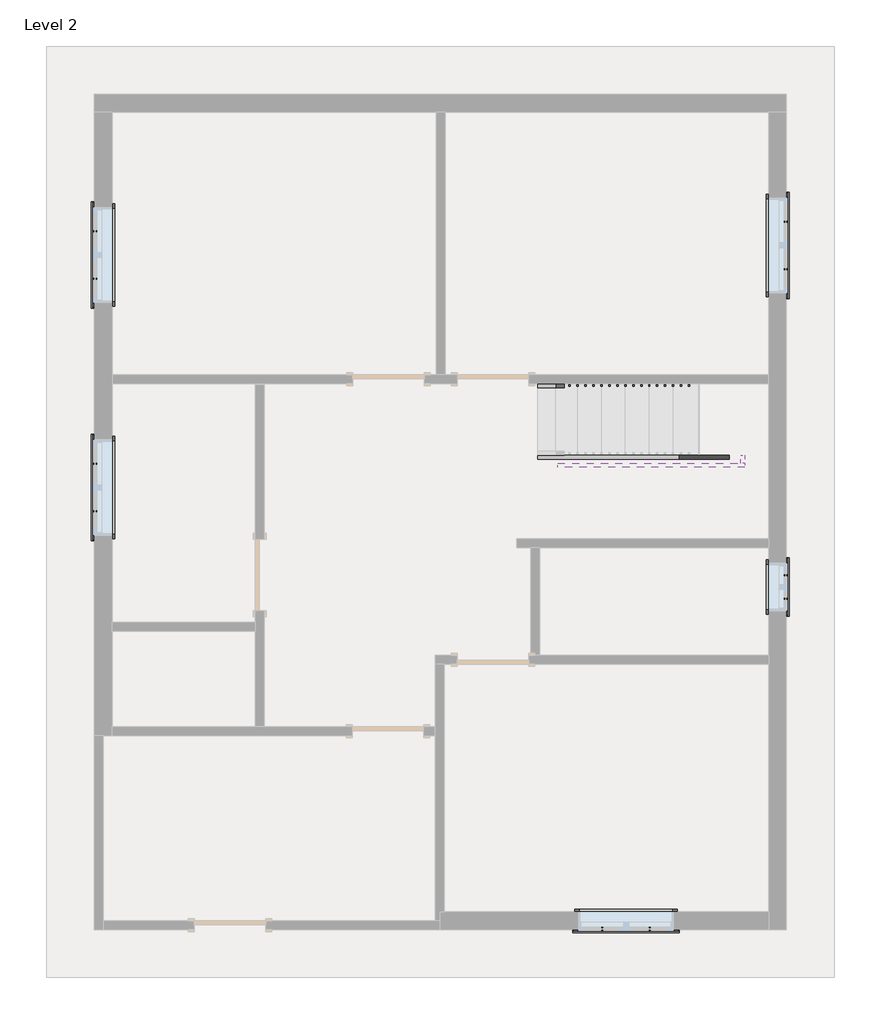
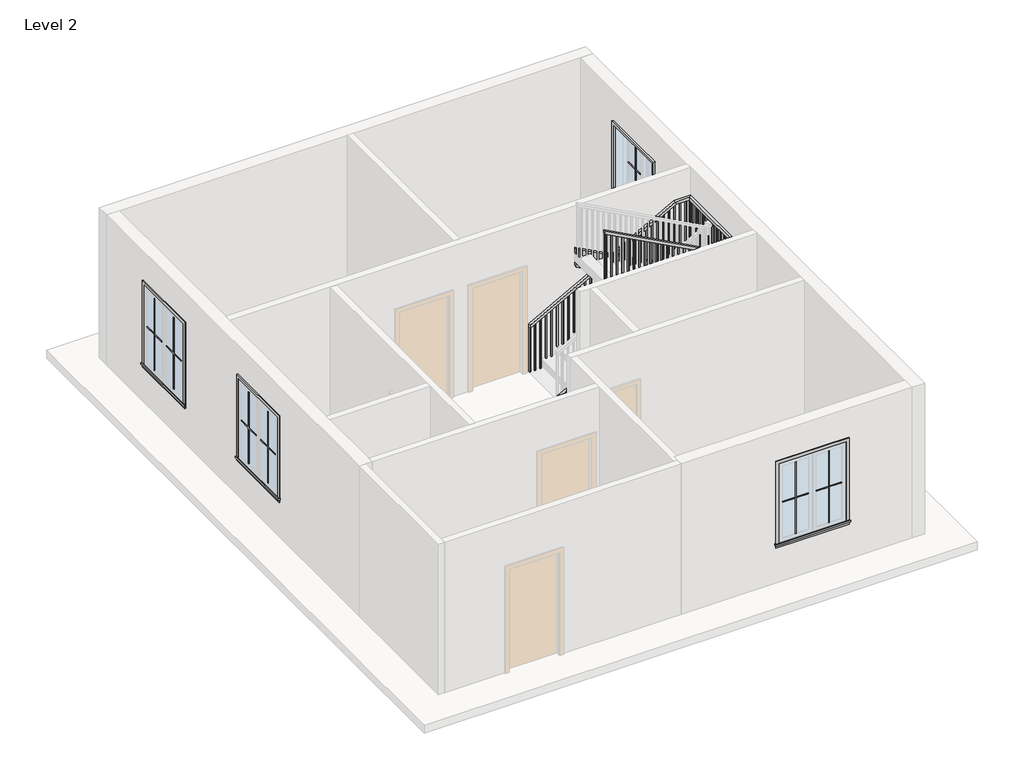
# One storey, part 2 of 2: 20 proxies, 3 members, 1 railing.
"""IFC4 building model written with IfcOpenShell, lengths in millimetres."""

from ifc_helpers import new_model, si_unit, frame, origin, place, context, project, spatial, polyline, outline, extrude, faceted_brep, transform, mapped, element, save
from components import muntin_pattern_2x2_muntin_pattern_2x2_6dad3731, muntin_pattern_2x2_muntin_pattern_2x2_a30a3345, muntin_pattern_2x2_muntin_pattern_2x2_53152e2c, muntin_pattern_2x2_muntin_pattern_2x2_e8f3e573, trim_window_exterior_flat_with_sill_92b9b949, trim_window_exterior_flat_with_sill_a665a915, trim_window_interior_flat_picture_frame_3bb882cf, trim_window_interior_flat_picture_frame_d485c387

model = new_model("IFC4")

# Units and contexts
model_context = context("Model", 3, world=origin())
ifc_project = project(units=[si_unit("LENGTHUNIT", "METRE", prefix="MILLI")], contexts=[model_context])

# Site, building, storey
site = spatial("IfcSite", under=ifc_project)
building = spatial("IfcBuilding", under=site)
storey = spatial("IfcBuildingStorey", under=building, Name="Level 2", Elevation=3048.0)

# Proxies
placement = place(None, origin())
muntin_pattern_2x2_muntin_pattern_2x2_shape = muntin_pattern_2x2_muntin_pattern_2x2_6dad3731(model_context)
element("IfcBuildingElementProxy", 1, Name="Muntin Pattern_2x2 : Muntin Pattern_2x2", ObjectType="Muntin Pattern_2x2 : Muntin Pattern_2x2", at=placement, inside=storey, context=model_context, shape_type="MappedRepresentation", body=[
    mapped(muntin_pattern_2x2_muntin_pattern_2x2_shape, transform((10003.63125, 2232.025, 4032.25), x_axis=(-1.0, 0.0, 0.0), y_axis=(0.0, -1.0, 0.0), z_axis=(0.0, 0.0, 1.0))),
])
element("IfcBuildingElementProxy", 2, Name="Muntin Pattern_2x2 : Muntin Pattern_2x2", ObjectType="Muntin Pattern_2x2 : Muntin Pattern_2x2", at=placement, inside=storey, context=model_context, shape_type="MappedRepresentation", body=[
    mapped(muntin_pattern_2x2_muntin_pattern_2x2_shape, transform((2917.825, 7567.6125, 4032.25), x_axis=(0.0, 1.0, 0.0), y_axis=(-1.0, 0.0, 0.0), z_axis=(0.0, 0.0, 1.0))),
])
element("IfcBuildingElementProxy", 3, Name="Muntin Pattern_2x2 : Muntin Pattern_2x2", ObjectType="Muntin Pattern_2x2 : Muntin Pattern_2x2", at=placement, inside=storey, context=model_context, shape_type="MappedRepresentation", body=[
    mapped(muntin_pattern_2x2_muntin_pattern_2x2_shape, transform((2917.825, 10536.2375, 4032.25), x_axis=(0.0, 1.0, 0.0), y_axis=(-1.0, 0.0, 0.0), z_axis=(0.0, 0.0, 1.0))),
])
element("IfcBuildingElementProxy", 4, Name="Muntin Pattern_2x2 : Muntin Pattern_2x2", ObjectType="Muntin Pattern_2x2 : Muntin Pattern_2x2", at=placement, inside=storey, context=model_context, shape_type="MappedRepresentation", body=[
    mapped(muntin_pattern_2x2_muntin_pattern_2x2_shape, transform((11737.975, 11264.9, 4032.25), x_axis=(0.0, -1.0, 0.0), y_axis=(1.0, 0.0, 0.0), z_axis=(0.0, 0.0, 1.0))),
])
muntin_pattern_2x2_muntin_pattern_2x2_2_shape = muntin_pattern_2x2_muntin_pattern_2x2_a30a3345(model_context)
element("IfcBuildingElementProxy", 5, Name="Muntin Pattern_2x2 : Muntin Pattern_2x2", ObjectType="Muntin Pattern_2x2 : Muntin Pattern_2x2", at=placement, inside=storey, context=model_context, shape_type="MappedRepresentation", body=[
    mapped(muntin_pattern_2x2_muntin_pattern_2x2_2_shape, transform((9397.20625, 2232.025, 4032.25), x_axis=(1.0, 0.0, 0.0), y_axis=(0.0, 1.0, 0.0), z_axis=(0.0, 0.0, 1.0))),
])
element("IfcBuildingElementProxy", 6, Name="Muntin Pattern_2x2 : Muntin Pattern_2x2", ObjectType="Muntin Pattern_2x2 : Muntin Pattern_2x2", at=placement, inside=storey, context=model_context, shape_type="MappedRepresentation", body=[
    mapped(muntin_pattern_2x2_muntin_pattern_2x2_2_shape, transform((2917.825, 8174.0375, 4032.25), x_axis=(0.0, -1.0, 0.0), y_axis=(1.0, 0.0, 0.0), z_axis=(0.0, 0.0, 1.0))),
])
element("IfcBuildingElementProxy", 7, Name="Muntin Pattern_2x2 : Muntin Pattern_2x2", ObjectType="Muntin Pattern_2x2 : Muntin Pattern_2x2", at=placement, inside=storey, context=model_context, shape_type="MappedRepresentation", body=[
    mapped(muntin_pattern_2x2_muntin_pattern_2x2_2_shape, transform((2917.825, 11142.6625, 4032.25), x_axis=(0.0, -1.0, 0.0), y_axis=(1.0, 0.0, 0.0), z_axis=(0.0, 0.0, 1.0))),
])
element("IfcBuildingElementProxy", 8, Name="Muntin Pattern_2x2 : Muntin Pattern_2x2", ObjectType="Muntin Pattern_2x2 : Muntin Pattern_2x2", at=placement, inside=storey, context=model_context, shape_type="MappedRepresentation", body=[
    mapped(muntin_pattern_2x2_muntin_pattern_2x2_2_shape, transform((11737.975, 10658.475, 4032.25), x_axis=(0.0, 1.0, 0.0), y_axis=(-1.0, 0.0, 0.0), z_axis=(0.0, 0.0, 1.0))),
])
muntin_pattern_2x2_muntin_pattern_2x2_3_shape = muntin_pattern_2x2_muntin_pattern_2x2_53152e2c(model_context)
element("IfcBuildingElementProxy", 9, Name="Muntin Pattern_2x2 : Muntin Pattern_2x2", ObjectType="Muntin Pattern_2x2 : Muntin Pattern_2x2", at=placement, inside=storey, context=model_context, shape_type="MappedRepresentation", body=[
    mapped(muntin_pattern_2x2_muntin_pattern_2x2_3_shape, transform((11737.975, 6748.4625, 4032.25), x_axis=(0.0, -1.0, 0.0), y_axis=(1.0, 0.0, 0.0), z_axis=(0.0, 0.0, 1.0))),
])
muntin_pattern_2x2_muntin_pattern_2x2_4_shape = muntin_pattern_2x2_muntin_pattern_2x2_e8f3e573(model_context)
element("IfcBuildingElementProxy", 10, Name="Muntin Pattern_2x2 : Muntin Pattern_2x2", ObjectType="Muntin Pattern_2x2 : Muntin Pattern_2x2", at=placement, inside=storey, context=model_context, shape_type="MappedRepresentation", body=[
    mapped(muntin_pattern_2x2_muntin_pattern_2x2_4_shape, transform((11737.975, 6446.8375, 4032.25), x_axis=(0.0, 1.0, 0.0), y_axis=(-1.0, 0.0, 0.0), z_axis=(0.0, 0.0, 1.0))),
])
trim_window_exterior_flat_with_sill_shape = trim_window_exterior_flat_with_sill_92b9b949(model_context)
element("IfcBuildingElementProxy", 11, Name="Trim-Window-Exterior-Flat : with Sill", ObjectType="Trim-Window-Exterior-Flat : with Sill", at=placement, inside=storey, context=model_context, shape_type="MappedRepresentation", body=[
    mapped(trim_window_exterior_flat_with_sill_shape, transform((9700.41875, 2222.5, 5486.4), x_axis=(1.0, 0.0, 0.0), y_axis=(0.0, 0.0, 1.0), z_axis=(0.0, -1.0, 0.0))),
])
element("IfcBuildingElementProxy", 12, Name="Trim-Window-Exterior-Flat : with Sill", ObjectType="Trim-Window-Exterior-Flat : with Sill", at=placement, inside=storey, context=model_context, shape_type="MappedRepresentation", body=[
    mapped(trim_window_exterior_flat_with_sill_shape, transform((2908.3, 7870.825, 5486.4), x_axis=(0.0, -1.0, 0.0), y_axis=(0.0, 0.0, 1.0), z_axis=(-1.0, 0.0, 0.0))),
])
element("IfcBuildingElementProxy", 13, Name="Trim-Window-Exterior-Flat : with Sill", ObjectType="Trim-Window-Exterior-Flat : with Sill", at=placement, inside=storey, context=model_context, shape_type="MappedRepresentation", body=[
    mapped(trim_window_exterior_flat_with_sill_shape, transform((2908.3, 10839.45, 5486.4), x_axis=(0.0, -1.0, 0.0), y_axis=(0.0, 0.0, 1.0), z_axis=(-1.0, 0.0, 0.0))),
])
element("IfcBuildingElementProxy", 14, Name="Trim-Window-Exterior-Flat : with Sill", ObjectType="Trim-Window-Exterior-Flat : with Sill", at=placement, inside=storey, context=model_context, shape_type="MappedRepresentation", body=[
    mapped(trim_window_exterior_flat_with_sill_shape, transform((11747.5, 10961.6875, 5486.4), x_axis=(0.0, 1.0, 0.0), y_axis=(0.0, 0.0, 1.0), z_axis=(1.0, 0.0, 0.0))),
])
trim_window_exterior_flat_with_sill_2_shape = trim_window_exterior_flat_with_sill_a665a915(model_context)
element("IfcBuildingElementProxy", 15, Name="Trim-Window-Exterior-Flat : with Sill", ObjectType="Trim-Window-Exterior-Flat : with Sill", at=placement, inside=storey, context=model_context, shape_type="MappedRepresentation", body=[
    mapped(trim_window_exterior_flat_with_sill_2_shape, transform((11747.5, 6597.65, 4876.8), x_axis=(0.0, 1.0, 0.0), y_axis=(0.0, 0.0, 1.0), z_axis=(1.0, 0.0, 0.0))),
])
trim_window_interior_flat_picture_frame_shape = trim_window_interior_flat_picture_frame_3bb882cf(model_context)
element("IfcBuildingElementProxy", 16, Name="Trim-Window-Interior-Flat : Picture Frame", ObjectType="Trim-Window-Interior-Flat : Picture Frame", at=placement, inside=storey, context=model_context, shape_type="MappedRepresentation", body=[
    mapped(trim_window_interior_flat_picture_frame_shape, transform((9700.41875, 2451.1, 5486.4), x_axis=(-1.0, 0.0, 0.0), y_axis=(0.0, 0.0, 1.0), z_axis=(0.0, 1.0, 0.0))),
])
element("IfcBuildingElementProxy", 17, Name="Trim-Window-Interior-Flat : Picture Frame", ObjectType="Trim-Window-Interior-Flat : Picture Frame", at=placement, inside=storey, context=model_context, shape_type="MappedRepresentation", body=[
    mapped(trim_window_interior_flat_picture_frame_shape, transform((3136.9, 7870.825, 5486.4), x_axis=(0.0, 1.0, 0.0), y_axis=(0.0, 0.0, 1.0), z_axis=(1.0, 0.0, 0.0))),
])
element("IfcBuildingElementProxy", 18, Name="Trim-Window-Interior-Flat : Picture Frame", ObjectType="Trim-Window-Interior-Flat : Picture Frame", at=placement, inside=storey, context=model_context, shape_type="MappedRepresentation", body=[
    mapped(trim_window_interior_flat_picture_frame_shape, transform((3136.9, 10839.45, 5486.4), x_axis=(0.0, 1.0, 0.0), y_axis=(0.0, 0.0, 1.0), z_axis=(1.0, 0.0, 0.0))),
])
element("IfcBuildingElementProxy", 19, Name="Trim-Window-Interior-Flat : Picture Frame", ObjectType="Trim-Window-Interior-Flat : Picture Frame", at=placement, inside=storey, context=model_context, shape_type="MappedRepresentation", body=[
    mapped(trim_window_interior_flat_picture_frame_shape, transform((11518.9, 10961.6875, 5486.4), x_axis=(0.0, -1.0, 0.0), y_axis=(0.0, 0.0, 1.0), z_axis=(-1.0, 0.0, 0.0))),
])
trim_window_interior_flat_picture_frame_2_shape = trim_window_interior_flat_picture_frame_d485c387(model_context)
element("IfcBuildingElementProxy", 20, Name="Trim-Window-Interior-Flat : Picture Frame", ObjectType="Trim-Window-Interior-Flat : Picture Frame", at=placement, inside=storey, context=model_context, shape_type="MappedRepresentation", body=[
    mapped(trim_window_interior_flat_picture_frame_2_shape, transform((11518.9, 6597.65, 4876.8), x_axis=(0.0, -1.0, 0.0), y_axis=(0.0, 0.0, 1.0), z_axis=(-1.0, 0.0, 0.0))),
])

# Members
element("IfcMember", 21, ObjectType="Stringer - 2\" Width", at=placement, inside=storey, context=model_context, shape_type="SweptSolid", body=[
    extrude(outline(polyline([(3292.4581083, 8572.5), (3048.0, 8572.5), (3048.0, 8761.9689927), (4325.1621978, 11163.3), (4670.3905183, 11163.3), (3292.4581083, 8572.5)])), frame((0.0, 8229.6, 0.0), z_axis=(0.0, 1.0, 0.0), x_axis=(0.0, 0.0, 1.0)), (0.0, 0.0, 1.0), 50.8),
])
element("IfcMember", 22, ObjectType="Stringer - 2\" Width", at=placement, inside=storey, context=model_context, shape_type="SweptSolid", body=[
    extrude(outline(polyline([(11163.3, 8280.4), (11214.1, 8280.4), (11214.1, 8178.8), (11163.3, 8178.8), (11163.3, 8280.4)])), frame((0.0, 0.0, 4423.6105263), z_axis=(0.0, 0.0, 1.0), x_axis=(1.0, 0.0, 0.0)), (0.0, 0.0, 1.0), 304.8),
])
element("IfcMember", 23, ObjectType="Stringer - 2\" Width", at=placement, inside=storey, context=model_context, shape_type="SweptSolid", body=[
    extrude(outline(polyline([(4512.9419568, 11214.1), (4857.380564, 11214.1), (6114.012143, 8826.5), (5769.5735358, 8826.5), (4512.9419568, 11214.1)])), frame((0.0, 8128.0, 0.0), z_axis=(0.0, 1.0, 0.0), x_axis=(0.0, 0.0, 1.0)), (0.0, 0.0, 1.0), 50.8),
])

# Railing
element("IfcRailing", 24, ObjectType="Handrail - Rectangular", at=placement, inside=storey, context=model_context, shape_type="SolidModel", body=[
    faceted_brep([(8572.5, 9194.8, 4122.8210526), (8572.5, 9194.8, 4064.9285199), (8572.5, 9144.0, 4064.9285199), (8572.5, 9144.0, 4122.8210526), (11214.1, 9194.8, 5566.6105263), (11227.076708, 9194.8, 5515.8105263), (11227.076708, 9144.0, 5515.8105263), (11214.1, 9144.0, 5566.6105263), (11518.9, 9194.8, 5566.6105263), (11518.9, 9194.8, 5515.8105263), (11468.1, 9144.0, 5515.8105263), (11468.1, 9144.0, 5566.6105263), (11518.9, 7340.6, 5566.6105263), (11518.9, 7289.8, 5515.8105263), (11468.1, 7289.8, 5515.8105263), (11468.1, 7340.6, 5566.6105263), (11518.9, 7340.6, 5631.4615901), (11518.9, 7289.8, 5580.6615901), (11468.1, 7289.8, 5580.6615901), (11468.1, 7340.6, 5631.4615901), (11518.9, 7213.6, 5631.4615901), (11518.9, 7213.6, 5580.6615901), (11468.1, 7264.4, 5580.6615901), (11468.1, 7264.4, 5631.4615901), (11391.9, 7213.6, 5631.4615901), (11379.1122768, 7213.6, 5580.6615901), (11379.1122768, 7264.4, 5580.6615901), (11391.9, 7264.4, 5631.4615901), (8826.5, 7213.6, 7010.4), (8826.5, 7264.4, 7010.4), (8826.5, 7264.4, 6952.7264198), (8826.5, 7213.6, 6952.7264198)], [[[0, 1, 2, 3]], [[1, 0, 4, 5]], [[2, 1, 5, 6]], [[3, 2, 6, 7]], [[0, 3, 7, 4]], [[5, 4, 8, 9]], [[6, 5, 9, 10]], [[7, 6, 10, 11]], [[4, 7, 11, 8]], [[9, 8, 12, 13]], [[10, 9, 13, 14]], [[11, 10, 14, 15]], [[8, 11, 15, 12]], [[13, 12, 16, 17]], [[14, 13, 17, 18]], [[15, 14, 18, 19]], [[12, 15, 19, 16]], [[17, 16, 20, 21]], [[18, 17, 21, 22]], [[19, 18, 22, 23]], [[16, 19, 23, 20]], [[21, 20, 24, 25]], [[22, 21, 25, 26]], [[23, 22, 26, 27]], [[20, 23, 27, 24]], [[28, 29, 30, 31]], [[25, 24, 28, 31]], [[26, 25, 31, 30]], [[27, 26, 30, 29]], [[24, 27, 29, 28]]]),
    extrude(outline(polyline([(6944.193385, 8842.375), (5935.5789474, 8842.375), (5935.5789474, 8861.425), (6933.9537434, 8861.425), (6944.193385, 8842.375)])), frame((0.0, 7229.475, 0.0), z_axis=(0.0, 1.0, 0.0), x_axis=(0.0, 0.0, 1.0)), (0.0, 0.0, 1.0), 19.05),
    extrude(outline(polyline([(6889.5819629, 8943.975), (5935.5789474, 8943.975), (5935.5789474, 8963.025), (6879.3423212, 8963.025), (6889.5819629, 8943.975)])), frame((0.0, 7229.475, 0.0), z_axis=(0.0, 1.0, 0.0), x_axis=(0.0, 0.0, 1.0)), (0.0, 0.0, 1.0), 19.05),
    extrude(outline(polyline([(6834.9705407, 9045.575), (5935.5789474, 9045.575), (5935.5789474, 9064.625), (6824.730899, 9064.625), (6834.9705407, 9045.575)])), frame((0.0, 7229.475, 0.0), z_axis=(0.0, 1.0, 0.0), x_axis=(0.0, 0.0, 1.0)), (0.0, 0.0, 1.0), 19.05),
    extrude(outline(polyline([(6780.3591185, 9147.175), (5775.1578947, 9147.175), (5775.1578947, 9166.225), (6770.1194769, 9166.225), (6780.3591185, 9147.175)])), frame((0.0, 7229.475, 0.0), z_axis=(0.0, 1.0, 0.0), x_axis=(0.0, 0.0, 1.0)), (0.0, 0.0, 1.0), 19.05),
    extrude(outline(polyline([(6725.7476964, 9248.775), (5775.1578947, 9248.775), (5775.1578947, 9267.825), (6715.5080547, 9267.825), (6725.7476964, 9248.775)])), frame((0.0, 7229.475, 0.0), z_axis=(0.0, 1.0, 0.0), x_axis=(0.0, 0.0, 1.0)), (0.0, 0.0, 1.0), 19.05),
    extrude(outline(polyline([(6671.1362742, 9350.375), (5775.1578947, 9350.375), (5775.1578947, 9369.425), (6660.8966325, 9369.425), (6671.1362742, 9350.375)])), frame((0.0, 7229.475, 0.0), z_axis=(0.0, 1.0, 0.0), x_axis=(0.0, 0.0, 1.0)), (0.0, 0.0, 1.0), 19.05),
    extrude(outline(polyline([(6616.524852, 9451.975), (5614.7368421, 9451.975), (5614.7368421, 9471.025), (6606.2852104, 9471.025), (6616.524852, 9451.975)])), frame((0.0, 7229.475, 0.0), z_axis=(0.0, 1.0, 0.0), x_axis=(0.0, 0.0, 1.0)), (0.0, 0.0, 1.0), 19.05),
    extrude(outline(polyline([(6561.9134298, 9553.575), (5614.7368421, 9553.575), (5614.7368421, 9572.625), (6551.6737882, 9572.625), (6561.9134298, 9553.575)])), frame((0.0, 7229.475, 0.0), z_axis=(0.0, 1.0, 0.0), x_axis=(0.0, 0.0, 1.0)), (0.0, 0.0, 1.0), 19.05),
    extrude(outline(polyline([(6507.3004835, 9655.175), (5614.7368421, 9655.175), (5614.7368421, 9674.225), (6496.8885402, 9674.225), (6507.3004835, 9655.175)])), frame((0.0, 7229.475, 0.0), z_axis=(0.0, 1.0, 0.0), x_axis=(0.0, 0.0, 1.0)), (0.0, 0.0, 1.0), 19.05),
    extrude(outline(polyline([(6452.6905855, 9756.775), (5454.3157895, 9756.775), (5454.3157895, 9775.825), (6442.4509438, 9775.825), (6452.6905855, 9756.775)])), frame((0.0, 7229.475, 0.0), z_axis=(0.0, 1.0, 0.0), x_axis=(0.0, 0.0, 1.0)), (0.0, 0.0, 1.0), 19.05),
    extrude(outline(polyline([(6398.0791633, 9858.375), (5454.3157895, 9858.375), (5454.3157895, 9877.425), (6387.8395217, 9877.425), (6398.0791633, 9858.375)])), frame((0.0, 7229.475, 0.0), z_axis=(0.0, 1.0, 0.0), x_axis=(0.0, 0.0, 1.0)), (0.0, 0.0, 1.0), 19.05),
    extrude(outline(polyline([(6343.4677411, 9959.975), (5454.3157895, 9959.975), (5454.3157895, 9979.025), (6333.2280995, 9979.025), (6343.4677411, 9959.975)])), frame((0.0, 7229.475, 0.0), z_axis=(0.0, 1.0, 0.0), x_axis=(0.0, 0.0, 1.0)), (0.0, 0.0, 1.0), 19.05),
    extrude(outline(polyline([(6288.856319, 10061.575), (5293.8947368, 10061.575), (5293.8947368, 10080.625), (6278.6166773, 10080.625), (6288.856319, 10061.575)])), frame((0.0, 7229.475, 0.0), z_axis=(0.0, 1.0, 0.0), x_axis=(0.0, 0.0, 1.0)), (0.0, 0.0, 1.0), 19.05),
    extrude(outline(polyline([(6234.2448968, 10163.175), (5293.8947368, 10163.175), (5293.8947368, 10182.225), (6224.0052551, 10182.225), (6234.2448968, 10163.175)])), frame((0.0, 7229.475, 0.0), z_axis=(0.0, 1.0, 0.0), x_axis=(0.0, 0.0, 1.0)), (0.0, 0.0, 1.0), 19.05),
    extrude(outline(polyline([(6179.6334746, 10264.775), (5293.8947368, 10264.775), (5293.8947368, 10283.825), (6169.393833, 10283.825), (6179.6334746, 10264.775)])), frame((0.0, 7229.475, 0.0), z_axis=(0.0, 1.0, 0.0), x_axis=(0.0, 0.0, 1.0)), (0.0, 0.0, 1.0), 19.05),
    extrude(outline(polyline([(6125.0220525, 10366.375), (5133.4736842, 10366.375), (5133.4736842, 10385.425), (6114.7824108, 10385.425), (6125.0220525, 10366.375)])), frame((0.0, 7229.475, 0.0), z_axis=(0.0, 1.0, 0.0), x_axis=(0.0, 0.0, 1.0)), (0.0, 0.0, 1.0), 19.05),
    extrude(outline(polyline([(6070.4106303, 10467.975), (5133.4736842, 10467.975), (5133.4736842, 10487.025), (6060.1709886, 10487.025), (6070.4106303, 10467.975)])), frame((0.0, 7229.475, 0.0), z_axis=(0.0, 1.0, 0.0), x_axis=(0.0, 0.0, 1.0)), (0.0, 0.0, 1.0), 19.05),
    extrude(outline(polyline([(6015.7992081, 10569.575), (5133.4736842, 10569.575), (5133.4736842, 10588.625), (6005.5595665, 10588.625), (6015.7992081, 10569.575)])), frame((0.0, 7229.475, 0.0), z_axis=(0.0, 1.0, 0.0), x_axis=(0.0, 0.0, 1.0)), (0.0, 0.0, 1.0), 19.05),
    extrude(outline(polyline([(5961.1877859, 10671.175), (4973.0526316, 10671.175), (4973.0526316, 10690.225), (5950.9481443, 10690.225), (5961.1877859, 10671.175)])), frame((0.0, 7229.475, 0.0), z_axis=(0.0, 1.0, 0.0), x_axis=(0.0, 0.0, 1.0)), (0.0, 0.0, 1.0), 19.05),
    extrude(outline(polyline([(5906.5763638, 10772.775), (4973.0526316, 10772.775), (4973.0526316, 10791.825), (5896.3367221, 10791.825), (5906.5763638, 10772.775)])), frame((0.0, 7229.475, 0.0), z_axis=(0.0, 1.0, 0.0), x_axis=(0.0, 0.0, 1.0)), (0.0, 0.0, 1.0), 19.05),
    extrude(outline(polyline([(5851.9649416, 10874.375), (4973.0526316, 10874.375), (4973.0526316, 10893.425), (5841.7252999, 10893.425), (5851.9649416, 10874.375)])), frame((0.0, 7229.475, 0.0), z_axis=(0.0, 1.0, 0.0), x_axis=(0.0, 0.0, 1.0)), (0.0, 0.0, 1.0), 19.05),
    extrude(outline(polyline([(5797.3535194, 10975.975), (4812.6315789, 10975.975), (4812.6315789, 10995.025), (5787.1138778, 10995.025), (5797.3535194, 10975.975)])), frame((0.0, 7229.475, 0.0), z_axis=(0.0, 1.0, 0.0), x_axis=(0.0, 0.0, 1.0)), (0.0, 0.0, 1.0), 19.05),
    extrude(outline(polyline([(5742.7420972, 11077.575), (4812.6315789, 11077.575), (4812.6315789, 11096.625), (5732.5024556, 11096.625), (5742.7420972, 11077.575)])), frame((0.0, 7229.475, 0.0), z_axis=(0.0, 1.0, 0.0), x_axis=(0.0, 0.0, 1.0)), (0.0, 0.0, 1.0), 19.05),
    extrude(outline(polyline([(5688.1306751, 11179.175), (4812.6315789, 11179.175), (4812.6315789, 11198.225), (5677.8910334, 11198.225), (5688.1306751, 11179.175)])), frame((0.0, 7229.475, 0.0), z_axis=(0.0, 1.0, 0.0), x_axis=(0.0, 0.0, 1.0)), (0.0, 0.0, 1.0), 19.05),
    extrude(outline(polyline([(5633.5192529, 11280.775), (4652.2105263, 11280.775), (4652.2105263, 11299.825), (5623.2796112, 11299.825), (5633.5192529, 11280.775)])), frame((0.0, 7229.475, 0.0), z_axis=(0.0, 1.0, 0.0), x_axis=(0.0, 0.0, 1.0)), (0.0, 0.0, 1.0), 19.05),
    extrude(outline(polyline([(5578.9078307, 11382.375), (4652.2105263, 11382.375), (4652.2105263, 11401.425), (5568.6681891, 11401.425), (5578.9078307, 11382.375)])), frame((0.0, 7229.475, 0.0), z_axis=(0.0, 1.0, 0.0), x_axis=(0.0, 0.0, 1.0)), (0.0, 0.0, 1.0), 19.05),
    extrude(outline(polyline([(11503.025, 7350.125), (11503.025, 7331.075), (11483.975, 7331.075), (11483.975, 7350.125), (11503.025, 7350.125)])), frame((0.0, 0.0, 4652.2105263), z_axis=(0.0, 0.0, 1.0), x_axis=(1.0, 0.0, 0.0)), (0.0, 0.0, 1.0), 863.6),
    extrude(outline(polyline([(11503.025, 7451.725), (11503.025, 7432.675), (11483.975, 7432.675), (11483.975, 7451.725), (11503.025, 7451.725)])), frame((0.0, 0.0, 4652.2105263), z_axis=(0.0, 0.0, 1.0), x_axis=(1.0, 0.0, 0.0)), (0.0, 0.0, 1.0), 863.6),
    extrude(outline(polyline([(11503.025, 7553.325), (11503.025, 7534.275), (11483.975, 7534.275), (11483.975, 7553.325), (11503.025, 7553.325)])), frame((0.0, 0.0, 4652.2105263), z_axis=(0.0, 0.0, 1.0), x_axis=(1.0, 0.0, 0.0)), (0.0, 0.0, 1.0), 863.6),
    extrude(outline(polyline([(11503.025, 7654.925), (11503.025, 7635.875), (11483.975, 7635.875), (11483.975, 7654.925), (11503.025, 7654.925)])), frame((0.0, 0.0, 4652.2105263), z_axis=(0.0, 0.0, 1.0), x_axis=(1.0, 0.0, 0.0)), (0.0, 0.0, 1.0), 863.6),
    extrude(outline(polyline([(11503.025, 7756.525), (11503.025, 7737.475), (11483.975, 7737.475), (11483.975, 7756.525), (11503.025, 7756.525)])), frame((0.0, 0.0, 4652.2105263), z_axis=(0.0, 0.0, 1.0), x_axis=(1.0, 0.0, 0.0)), (0.0, 0.0, 1.0), 863.6),
    extrude(outline(polyline([(11503.025, 7858.125), (11503.025, 7839.075), (11483.975, 7839.075), (11483.975, 7858.125), (11503.025, 7858.125)])), frame((0.0, 0.0, 4652.2105263), z_axis=(0.0, 0.0, 1.0), x_axis=(1.0, 0.0, 0.0)), (0.0, 0.0, 1.0), 863.6),
    extrude(outline(polyline([(11503.025, 7959.725), (11503.025, 7940.675), (11483.975, 7940.675), (11483.975, 7959.725), (11503.025, 7959.725)])), frame((0.0, 0.0, 4652.2105263), z_axis=(0.0, 0.0, 1.0), x_axis=(1.0, 0.0, 0.0)), (0.0, 0.0, 1.0), 863.6),
    extrude(outline(polyline([(11503.025, 8061.325), (11503.025, 8042.275), (11483.975, 8042.275), (11483.975, 8061.325), (11503.025, 8061.325)])), frame((0.0, 0.0, 4652.2105263), z_axis=(0.0, 0.0, 1.0), x_axis=(1.0, 0.0, 0.0)), (0.0, 0.0, 1.0), 863.6),
    extrude(outline(polyline([(11503.025, 8162.925), (11503.025, 8143.875), (11483.975, 8143.875), (11483.975, 8162.925), (11503.025, 8162.925)])), frame((0.0, 0.0, 4652.2105263), z_axis=(0.0, 0.0, 1.0), x_axis=(1.0, 0.0, 0.0)), (0.0, 0.0, 1.0), 863.6),
    extrude(outline(polyline([(11503.025, 8264.525), (11503.025, 8245.475), (11483.975, 8245.475), (11483.975, 8264.525), (11503.025, 8264.525)])), frame((0.0, 0.0, 4652.2105263), z_axis=(0.0, 0.0, 1.0), x_axis=(1.0, 0.0, 0.0)), (0.0, 0.0, 1.0), 863.6),
    extrude(outline(polyline([(11503.025, 8366.125), (11503.025, 8347.075), (11483.975, 8347.075), (11483.975, 8366.125), (11503.025, 8366.125)])), frame((0.0, 0.0, 4652.2105263), z_axis=(0.0, 0.0, 1.0), x_axis=(1.0, 0.0, 0.0)), (0.0, 0.0, 1.0), 863.6),
    extrude(outline(polyline([(11503.025, 8467.725), (11503.025, 8448.675), (11483.975, 8448.675), (11483.975, 8467.725), (11503.025, 8467.725)])), frame((0.0, 0.0, 4652.2105263), z_axis=(0.0, 0.0, 1.0), x_axis=(1.0, 0.0, 0.0)), (0.0, 0.0, 1.0), 863.6),
    extrude(outline(polyline([(11503.025, 8569.325), (11503.025, 8550.275), (11483.975, 8550.275), (11483.975, 8569.325), (11503.025, 8569.325)])), frame((0.0, 0.0, 4652.2105263), z_axis=(0.0, 0.0, 1.0), x_axis=(1.0, 0.0, 0.0)), (0.0, 0.0, 1.0), 863.6),
    extrude(outline(polyline([(11503.025, 8670.925), (11503.025, 8651.875), (11483.975, 8651.875), (11483.975, 8670.925), (11503.025, 8670.925)])), frame((0.0, 0.0, 4652.2105263), z_axis=(0.0, 0.0, 1.0), x_axis=(1.0, 0.0, 0.0)), (0.0, 0.0, 1.0), 863.6),
    extrude(outline(polyline([(11503.025, 8772.525), (11503.025, 8753.475), (11483.975, 8753.475), (11483.975, 8772.525), (11503.025, 8772.525)])), frame((0.0, 0.0, 4652.2105263), z_axis=(0.0, 0.0, 1.0), x_axis=(1.0, 0.0, 0.0)), (0.0, 0.0, 1.0), 863.6),
    extrude(outline(polyline([(11503.025, 8874.125), (11503.025, 8855.075), (11483.975, 8855.075), (11483.975, 8874.125), (11503.025, 8874.125)])), frame((0.0, 0.0, 4652.2105263), z_axis=(0.0, 0.0, 1.0), x_axis=(1.0, 0.0, 0.0)), (0.0, 0.0, 1.0), 863.6),
    extrude(outline(polyline([(11503.025, 8975.725), (11503.025, 8956.675), (11483.975, 8956.675), (11483.975, 8975.725), (11503.025, 8975.725)])), frame((0.0, 0.0, 4652.2105263), z_axis=(0.0, 0.0, 1.0), x_axis=(1.0, 0.0, 0.0)), (0.0, 0.0, 1.0), 863.6),
    extrude(outline(polyline([(11503.025, 9077.325), (11503.025, 9058.275), (11483.975, 9058.275), (11483.975, 9077.325), (11503.025, 9077.325)])), frame((0.0, 0.0, 4652.2105263), z_axis=(0.0, 0.0, 1.0), x_axis=(1.0, 0.0, 0.0)), (0.0, 0.0, 1.0), 863.6),
    extrude(outline(polyline([(11407.775, 9178.925), (11426.825, 9178.925), (11426.825, 9159.875), (11407.775, 9159.875), (11407.775, 9178.925)])), frame((0.0, 0.0, 4652.2105263), z_axis=(0.0, 0.0, 1.0), x_axis=(1.0, 0.0, 0.0)), (0.0, 0.0, 1.0), 863.6),
    extrude(outline(polyline([(11306.175, 9178.925), (11325.225, 9178.925), (11325.225, 9159.875), (11306.175, 9159.875), (11306.175, 9178.925)])), frame((0.0, 0.0, 4652.2105263), z_axis=(0.0, 0.0, 1.0), x_axis=(1.0, 0.0, 0.0)), (0.0, 0.0, 1.0), 863.6),
    extrude(outline(polyline([(5503.512022, 11204.575), (4652.2105263, 11204.575), (4652.2105263, 11223.625), (5513.9239653, 11223.625), (5503.512022, 11204.575)])), frame((0.0, 9159.875, 0.0), z_axis=(0.0, 1.0, 0.0), x_axis=(0.0, 0.0, 1.0)), (0.0, 0.0, 1.0), 19.05),
    extrude(outline(polyline([(5447.9816576, 11102.975), (4491.7894737, 11102.975), (4491.7894737, 11122.025), (5458.3936009, 11122.025), (5447.9816576, 11102.975)])), frame((0.0, 9159.875, 0.0), z_axis=(0.0, 1.0, 0.0), x_axis=(0.0, 0.0, 1.0)), (0.0, 0.0, 1.0), 19.05),
    extrude(outline(polyline([(5392.4512932, 11001.375), (4491.7894737, 11001.375), (4491.7894737, 11020.425), (5402.8632365, 11020.425), (5392.4512932, 11001.375)])), frame((0.0, 9159.875, 0.0), z_axis=(0.0, 1.0, 0.0), x_axis=(0.0, 0.0, 1.0)), (0.0, 0.0, 1.0), 19.05),
    extrude(outline(polyline([(5336.9209288, 10899.775), (4491.7894737, 10899.775), (4491.7894737, 10918.825), (5347.3328722, 10918.825), (5336.9209288, 10899.775)])), frame((0.0, 9159.875, 0.0), z_axis=(0.0, 1.0, 0.0), x_axis=(0.0, 0.0, 1.0)), (0.0, 0.0, 1.0), 19.05),
    extrude(outline(polyline([(5281.3905645, 10798.175), (4331.3684211, 10798.175), (4331.3684211, 10817.225), (5291.8025078, 10817.225), (5281.3905645, 10798.175)])), frame((0.0, 9159.875, 0.0), z_axis=(0.0, 1.0, 0.0), x_axis=(0.0, 0.0, 1.0)), (0.0, 0.0, 1.0), 19.05),
    extrude(outline(polyline([(5225.8602001, 10696.575), (4331.3684211, 10696.575), (4331.3684211, 10715.625), (5236.2721434, 10715.625), (5225.8602001, 10696.575)])), frame((0.0, 9159.875, 0.0), z_axis=(0.0, 1.0, 0.0), x_axis=(0.0, 0.0, 1.0)), (0.0, 0.0, 1.0), 19.05),
    extrude(outline(polyline([(5170.3298357, 10594.975), (4331.3684211, 10594.975), (4331.3684211, 10614.025), (5180.741779, 10614.025), (5170.3298357, 10594.975)])), frame((0.0, 9159.875, 0.0), z_axis=(0.0, 1.0, 0.0), x_axis=(0.0, 0.0, 1.0)), (0.0, 0.0, 1.0), 19.05),
    extrude(outline(polyline([(5114.7994714, 10493.375), (4170.9473684, 10493.375), (4170.9473684, 10512.425), (5125.2114147, 10512.425), (5114.7994714, 10493.375)])), frame((0.0, 9159.875, 0.0), z_axis=(0.0, 1.0, 0.0), x_axis=(0.0, 0.0, 1.0)), (0.0, 0.0, 1.0), 19.05),
    extrude(outline(polyline([(5059.269107, 10391.775), (4170.9473684, 10391.775), (4170.9473684, 10410.825), (5069.6810503, 10410.825), (5059.269107, 10391.775)])), frame((0.0, 9159.875, 0.0), z_axis=(0.0, 1.0, 0.0), x_axis=(0.0, 0.0, 1.0)), (0.0, 0.0, 1.0), 19.05),
    extrude(outline(polyline([(5003.7387426, 10290.175), (4170.9473684, 10290.175), (4170.9473684, 10309.225), (5014.1506859, 10309.225), (5003.7387426, 10290.175)])), frame((0.0, 9159.875, 0.0), z_axis=(0.0, 1.0, 0.0), x_axis=(0.0, 0.0, 1.0)), (0.0, 0.0, 1.0), 19.05),
    extrude(outline(polyline([(4948.2083782, 10188.575), (4010.5263158, 10188.575), (4010.5263158, 10207.625), (4958.6203216, 10207.625), (4948.2083782, 10188.575)])), frame((0.0, 9159.875, 0.0), z_axis=(0.0, 1.0, 0.0), x_axis=(0.0, 0.0, 1.0)), (0.0, 0.0, 1.0), 19.05),
    extrude(outline(polyline([(4892.6780139, 10086.975), (4010.5263158, 10086.975), (4010.5263158, 10106.025), (4903.0899572, 10106.025), (4892.6780139, 10086.975)])), frame((0.0, 9159.875, 0.0), z_axis=(0.0, 1.0, 0.0), x_axis=(0.0, 0.0, 1.0)), (0.0, 0.0, 1.0), 19.05),
    extrude(outline(polyline([(4837.1476495, 9985.375), (4010.5263158, 9985.375), (4010.5263158, 10004.425), (4847.5595928, 10004.425), (4837.1476495, 9985.375)])), frame((0.0, 9159.875, 0.0), z_axis=(0.0, 1.0, 0.0), x_axis=(0.0, 0.0, 1.0)), (0.0, 0.0, 1.0), 19.05),
    extrude(outline(polyline([(4781.6172851, 9883.775), (3850.1052632, 9883.775), (3850.1052632, 9902.825), (4792.0292284, 9902.825), (4781.6172851, 9883.775)])), frame((0.0, 9159.875, 0.0), z_axis=(0.0, 1.0, 0.0), x_axis=(0.0, 0.0, 1.0)), (0.0, 0.0, 1.0), 19.05),
    extrude(outline(polyline([(4726.0869207, 9782.175), (3850.1052632, 9782.175), (3850.1052632, 9801.225), (4736.4988641, 9801.225), (4726.0869207, 9782.175)])), frame((0.0, 9159.875, 0.0), z_axis=(0.0, 1.0, 0.0), x_axis=(0.0, 0.0, 1.0)), (0.0, 0.0, 1.0), 19.05),
    extrude(outline(polyline([(4670.5565564, 9680.575), (3850.1052632, 9680.575), (3850.1052632, 9699.625), (4680.9684997, 9699.625), (4670.5565564, 9680.575)])), frame((0.0, 9159.875, 0.0), z_axis=(0.0, 1.0, 0.0), x_axis=(0.0, 0.0, 1.0)), (0.0, 0.0, 1.0), 19.05),
    extrude(outline(polyline([(4615.026192, 9578.975), (3689.6842105, 9578.975), (3689.6842105, 9598.025), (4625.4381353, 9598.025), (4615.026192, 9578.975)])), frame((0.0, 9159.875, 0.0), z_axis=(0.0, 1.0, 0.0), x_axis=(0.0, 0.0, 1.0)), (0.0, 0.0, 1.0), 19.05),
    extrude(outline(polyline([(4559.4958276, 9477.375), (3689.6842105, 9477.375), (3689.6842105, 9496.425), (4569.9077709, 9496.425), (4559.4958276, 9477.375)])), frame((0.0, 9159.875, 0.0), z_axis=(0.0, 1.0, 0.0), x_axis=(0.0, 0.0, 1.0)), (0.0, 0.0, 1.0), 19.05),
    extrude(outline(polyline([(4503.9654633, 9375.775), (3689.6842105, 9375.775), (3689.6842105, 9394.825), (4514.3774066, 9394.825), (4503.9654633, 9375.775)])), frame((0.0, 9159.875, 0.0), z_axis=(0.0, 1.0, 0.0), x_axis=(0.0, 0.0, 1.0)), (0.0, 0.0, 1.0), 19.05),
    extrude(outline(polyline([(4448.4350989, 9274.175), (3529.2631579, 9274.175), (3529.2631579, 9293.225), (4458.8470422, 9293.225), (4448.4350989, 9274.175)])), frame((0.0, 9159.875, 0.0), z_axis=(0.0, 1.0, 0.0), x_axis=(0.0, 0.0, 1.0)), (0.0, 0.0, 1.0), 19.05),
    extrude(outline(polyline([(4392.9047345, 9172.575), (3529.2631579, 9172.575), (3529.2631579, 9191.625), (4403.3166778, 9191.625), (4392.9047345, 9172.575)])), frame((0.0, 9159.875, 0.0), z_axis=(0.0, 1.0, 0.0), x_axis=(0.0, 0.0, 1.0)), (0.0, 0.0, 1.0), 19.05),
    extrude(outline(polyline([(4337.3743701, 9070.975), (3529.2631579, 9070.975), (3529.2631579, 9090.025), (4347.7863135, 9090.025), (4337.3743701, 9070.975)])), frame((0.0, 9159.875, 0.0), z_axis=(0.0, 1.0, 0.0), x_axis=(0.0, 0.0, 1.0)), (0.0, 0.0, 1.0), 19.05),
    extrude(outline(polyline([(4281.8440058, 8969.375), (3368.8421053, 8969.375), (3368.8421053, 8988.425), (4292.2559491, 8988.425), (4281.8440058, 8969.375)])), frame((0.0, 9159.875, 0.0), z_axis=(0.0, 1.0, 0.0), x_axis=(0.0, 0.0, 1.0)), (0.0, 0.0, 1.0), 19.05),
    extrude(outline(polyline([(4226.3136414, 8867.775), (3368.8421053, 8867.775), (3368.8421053, 8886.825), (4236.7255847, 8886.825), (4226.3136414, 8867.775)])), frame((0.0, 9159.875, 0.0), z_axis=(0.0, 1.0, 0.0), x_axis=(0.0, 0.0, 1.0)), (0.0, 0.0, 1.0), 19.05),
    extrude(outline(polyline([(4170.783277, 8766.175), (3208.4210526, 8766.175), (3208.4210526, 8785.225), (4181.1952203, 8785.225), (4170.783277, 8766.175)])), frame((0.0, 9159.875, 0.0), z_axis=(0.0, 1.0, 0.0), x_axis=(0.0, 0.0, 1.0)), (0.0, 0.0, 1.0), 19.05),
    extrude(outline(polyline([(4115.2529126, 8664.575), (3208.4210526, 8664.575), (3208.4210526, 8683.625), (4125.664856, 8683.625), (4115.2529126, 8664.575)])), frame((0.0, 9159.875, 0.0), z_axis=(0.0, 1.0, 0.0), x_axis=(0.0, 0.0, 1.0)), (0.0, 0.0, 1.0), 19.05),
    extrude(outline(polyline([(11503.025, 7248.525), (11503.025, 7229.475), (11483.975, 7229.475), (11483.975, 7248.525), (11503.025, 7248.525)])), frame((0.0, 0.0, 4652.2105263), z_axis=(0.0, 0.0, 1.0), x_axis=(1.0, 0.0, 0.0)), (0.0, 0.0, 1.0), 928.4510638),
    extrude(outline(polyline([(11483.975, 9178.925), (11503.025, 9178.925), (11503.025, 9159.875), (11483.975, 9159.875), (11483.975, 9178.925)])), frame((0.0, 0.0, 4652.2105263), z_axis=(0.0, 0.0, 1.0), x_axis=(1.0, 0.0, 0.0)), (0.0, 0.0, 1.0), 863.6),
    extrude(outline(polyline([(6952.7264198, 8826.5), (5935.5789474, 8826.5), (5935.5789474, 8845.55), (6942.4867781, 8845.55), (6952.7264198, 8826.5)])), frame((0.0, 7229.475, 0.0), z_axis=(0.0, 1.0, 0.0), x_axis=(0.0, 0.0, 1.0)), (0.0, 0.0, 1.0), 19.05),
    extrude(outline(polyline([(4064.9285199, 8572.5), (3208.4210526, 8572.5), (3208.4210526, 8591.55), (4075.3404633, 8591.55), (4064.9285199, 8572.5)])), frame((0.0, 9159.875, 0.0), z_axis=(0.0, 1.0, 0.0), x_axis=(0.0, 0.0, 1.0)), (0.0, 0.0, 1.0), 19.05),
])

save(model, "model.ifc")

# Revit data of these elements
# Type "Muntin Pattern_2x2 : Muntin Pattern_2x2"
#   Width [instance default] = 4' - 0"
#   Thickness = 0' - 0 1/2"
#   Height [instance default] = 4' - 0"
#   Distance = 0' - 0 3/4"
#   Interior Material [instance default] = none
#   Exterior Material [instance default] = none
#   Default Elevation = 0
# Type "Trim-Window-Exterior-Flat : with Sill"
#   Trim Width = 0' - 2 1/4"
#   Trim Thickness_Picture Frame = 0' - 1 1/4"
#   Trim Thickness_with Sill = 0' - 0 3/4"
#   Sill Thickness = 0' - 1 1/4"
#   Opening Width [instance default] = 2' - 0"
#   Opening Height [instance default] = 3' - 0"
#   Default Elevation = 4' - 0"
#   Sill = yes
#   Picture Frame = no
#   Trim Material [instance default] = none
# Type "Trim-Window-Interior-Flat : Picture Frame"
#   Trim Thickness_Picture Frame = 0' - 1 1/4"
#   Trim Width = 0' - 2 1/4"
#   Trim Thickness_with Sill = 0' - 0 3/4"
#   Sill Thickness = 0' - 1 1/4"
#   Opening Width [instance default] = 2' - 0"
#   Opening Height [instance default] = 3' - 0"
#   Default Elevation = 4' - 0"
#   Sill = no
#   Picture Frame = yes
#   Trim Material [instance default] = none
# Type "Handrail - Rectangular"
#   Assembly Code = "C2010400"
#   built-in parameter 1008612 = 0.0416667 (stored number, unit not read)
#   built-in parameter 1008611 = 0.0416667 (stored number, unit not read)
#   built-in parameter 1008609 = 0.333333 (stored number, unit not read)
#   built-in parameter 1008604 = 0.166667 (stored number, unit not read)
#   built-in parameter 1008603 = 0.166667 (stored number, unit not read)
#   Railing Height = 3' - 0"
#   built-in parameter 1008630 = 2
#   built-in parameter 1008610 = 2
#   built-in parameter 1008618 = Baluster - Square : 3/4"
# Elements 1, 2, 3, 4, 5, 6, 7, 8 (IfcBuildingElementProxy, "Muntin Pattern_2x2 : Muntin Pattern_2x2")
#   Width = 1' - 6 5/8"
#   Height = 4' - 6 1/2"
#   Interior Material = Wood - Stained
#   Exterior Material = Clad - White
#   Phase Created = New Construction
#   Materials on its faces: "Clad - White", "Wood - Stained"
# Elements 9, 10 (IfcBuildingElementProxy, "Muntin Pattern_2x2 : Muntin Pattern_2x2")
#   Width = 0' - 6 5/8"
#   Height = 2' - 6 1/2"
#   Interior Material = Wood - Stained
#   Exterior Material = Clad - White
#   Phase Created = New Construction
#   Materials on its faces: "Clad - White", "Wood - Stained"
# Elements 11, 12, 13, 14 (IfcBuildingElementProxy, "Trim-Window-Exterior-Flat : with Sill")
#   Opening Width = 4' - 0"
#   Opening Height = 5' - 0"
#   Trim Material = Clad - White
#   Phase Created = New Construction
#   Materials on its faces: "Clad - White"
# Element 15 (IfcBuildingElementProxy, "Trim-Window-Exterior-Flat : with Sill")
#   Opening Width = 2' - 0"
#   Opening Height = 3' - 0"
#   Trim Material = Clad - White
#   Phase Created = New Construction
#   Materials on its faces: "Clad - White"
# Elements 16, 17, 18, 19 (IfcBuildingElementProxy, "Trim-Window-Interior-Flat : Picture Frame")
#   Opening Width = 4' - 0"
#   Opening Height = 5' - 0"
#   Trim Material = Wood - Stained
#   Phase Created = New Construction
#   Materials on its faces: "Wood - Stained"
# Element 20 (IfcBuildingElementProxy, "Trim-Window-Interior-Flat : Picture Frame")
#   Opening Width = 2' - 0"
#   Opening Height = 3' - 0"
#   Trim Material = Wood - Stained
#   Phase Created = New Construction
#   Materials on its faces: "Wood - Stained"
# Elements 21, 22, 23 (IfcMember, "Stringer - 2\" Width")
#   Phase Created = New Construction
# Element 24 (IfcRailing, "Handrail - Rectangular")
#   Phase Created = New Construction
# Materials
#   "Clad - White": class "Wood", colour RGB 242 242 238, transparency 0, Cost = 0
#   "Wood - Stained": class "Wood", colour RGB 224 178 126, transparency 0, Cost = 0
